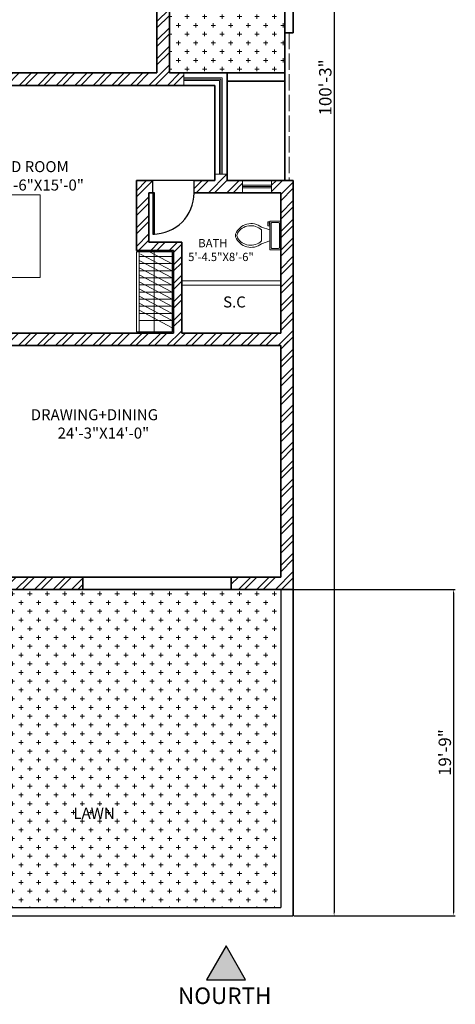
# Model space of a CAD drawing. Units: inches. Extents: x 839 to 1638, y 2998 to 4342.
# Tile 2 of 4: x 1321 to 1638, y 2998 to 3713. Entities that reach past the tile are written whole.
import ezdxf

# ---------------------------------------------------------------- set-up
doc = ezdxf.new("R2010")
doc.units = ezdxf.units.IN
doc.linetypes.add('ACAD_ISO02W100', pattern=[15, 12, -3])
for name, color, linetype, lineweight in [('A-ANNO-DIMS', 2, 'Continuous', 18), ('A-ANNO-SYMB', 7, 'Continuous', 25), ('A-AREA-IDEN', 7, 'Continuous', 18), ('A-DOOR', 4, 'Continuous', 25), ('A-DOOR-JAMB', 7, 'Continuous', 25), ('A-FLOR-CASE', 9, 'Continuous', 20), ('A-FLOR-CASE-PATT', 252, 'Continuous', 13), ('A-FLOR-FIXT', 9, 'Continuous', 18), ('A-FLOR-OVHD', 8, 'ACAD_ISO02W100', 18), ('A-FURN', 8, 'Continuous', 18), ('A-WALL', 7, 'Continuous', 35), ('A-WALL-PATT', 252, 'Continuous', 13), ('C-PROP', 7, 'Continuous', 30)]:
    doc.layers.add(name, color=color, linetype=linetype, lineweight=lineweight)
doc.layers.add('A-GLAZ', color=244, linetype='Continuous', lineweight=20, true_color=0x991b1e)
doc.layers.add('L-SITE-PATT', color=116, linetype='Continuous', lineweight=13, true_color=0x136734)
doc.styles.get("Standard").update_dxf_attribs({"font": 'arial.ttf'})
doc.dimstyles.new('ISO-25', dxfattribs={"dimtxt": 9, "dimasz": 2.5, "dimexe": 1.25, "dimexo": 0.625, "dimtad": 1, "dimlunit": 3, "dimtxsty": 'Standard', "dimcen": 2.5, "dimadec": 0, "dimazin": 0, "dimtfac": 1, "dimtmove": 0, "dimatfit": 3, "dimfxl": 1, "dimarcsym": 0})

# ---------------------------------------------------------------- blocks, each defined once
blk = doc.blocks.new('*U4')
for p, q in [((0, 0), (0, 6)), ((40, 0), (40, 6))]:
    blk.add_line(p, q)
blk.add_lwpolyline([(0, 0), (0, -40), (1.75, -40), (1.75, 0)], close=True)
blk.add_arc((0, 0), 40, 270, 0)
blk = doc.blocks.new('*U15')
for p, q in [((9.5, -6), (9.5, -2)), ((-10, -8.5), (-8, -8.5)), ((-10, -9.5), (-10, -8.5)), ((-7, -9.5), (-10, -9.5)), ((-8, -8.5), (-8, -8)), ((-7, -8), (-7, -9.5)), ((-4, -8), (-6, -14)), ((4, -14), (-4, -14)), ((4, -8), (6, -14))]:
    blk.add_line(p, q)
blk.add_lwpolyline([(10.5, -8), (10.5, 0), (-10.5, 0), (-10.5, -8)], close=True)
for points in [[(-9.5, -2), (-9.5, -6)], [(8.5, -1), (-8.5, -1)], [(-8.5, -7), (8.5, -7)]]:
    blk.add_lwpolyline(points)
for centre, radius, start, end in [((-8.62, -1.88), 0.884, 81.8699, 188.1301), ((-8.62, -6.12), 0.884, 171.8699, 278.1301), ((8.62, -1.88), 0.884, 351.8699, 98.1301), ((8.62, -6.12), 0.884, 261.8699, 8.1301), ((3.52, -21.58), 12.17, 141.46911, 247.97143), ((4.2, -21.82), 11.33, 136.36773, 238.94682), ((-3.52, -21.58), 12.17, 292.02843, 38.53071), ((-4.2, -21.82), 11.33, 301.05301, 43.63209), ((0, -27.88), 4, 245.73182, 294.26817), ((0, -29), 4, 254.86053, 285.13947)]:
    blk.add_arc(centre, radius, start, end)
blk = doc.blocks.new('Bed - Queen')
for p, q in [((0, -80.00003), (0, 0)), ((0, 0), (59.99999, 0)), ((59.99999, 0), (59.99999, -80.00003)), ((7.99999, -1.2), (28.79998, -1.2)), ((7.99999, -14.4), (7.99999, -1.2)), ((28.79998, -1.2), (28.79998, -14.4)), ((31.19999, -1.2), (51.99999, -1.2)), ((31.19999, -14.4), (31.19999, -1.2)), ((51.99999, -1.2), (51.99999, -16.4)), ((0, -14.4), (44.8, -14.4)), ((44.8, -16.8), (0, -16.8)), ((59.99999, -29.6), (44.8, -14.4)), ((44.8, -14.4), (44.8, -29.6)), ((51.99999, -16.4), (46.79936, -16.4)), ((44.8, -29.6), (59.99999, -29.6)), ((59.99999, -80.00003), (0, -80.00003))]:
    blk.add_line(p, q)
blk = doc.blocks.new('*D21')
at = {"layer": 'A-ANNO-DIMS', "color": 0, "lineweight": -2, "transparency": 16777216}
for p, q in [((1520.79, 4264.84), (1551.14, 4264.84)), ((1549.89, 4262.34), (1549.89, 3064.34)), ((1520.79, 3061.84), (1551.14, 3061.84))]:
    blk.add_line(p, q, dxfattribs=at)
at = {"layer": 'A-ANNO-DIMS', "color": 0, "transparency": 16777216}
for points in [[(1549.48, 4262.34), (1550.31, 4262.34), (1549.89, 4264.84)], [(1549.48, 3064.34), (1550.31, 3064.34), (1549.89, 3061.84)]]:
    blk.add_solid(points, dxfattribs=at)
at = {"layer": 'Defpoints', "color": 0, "transparency": 16777216}
for p in [(1520.17, 4264.84), (1520.17, 3061.84), (1549.89, 3061.84)]:
    blk.add_point(p, dxfattribs=at)
at = {"layer": 'A-ANNO-DIMS', "color": 0, "transparency": 16777216, "insert": (1544.67, 3663.34), "char_height": 9, "attachment_point": 5, "rotation": 90}
blk.add_mtext('100\'-3"', dxfattribs=at)
blk = doc.blocks.new('WIN-21x9')
for p, q in [((0, 5.5), (21, 5.5)), ((0, 4.5), (21, 4.5)), ((0, 3.5), (21, 3.5))]:
    blk.add_line(p, q)
blk.add_lwpolyline([(0, 9), (21, 9), (21, 0), (0, 0)], close=True)
blk = doc.blocks.new('*D51')
at = {"layer": 'A-ANNO-DIMS', "color": 0, "lineweight": -2, "transparency": 16777216}
for p, q in [((1520.79, 3298.84), (1638.02, 3298.84)), ((1636.77, 3296.34), (1636.77, 3064.34)), ((1520.79, 3061.84), (1638.02, 3061.84))]:
    blk.add_line(p, q, dxfattribs=at)
at = {"layer": 'A-ANNO-DIMS', "color": 0, "transparency": 16777216}
for points in [[(1636.35, 3296.34), (1637.19, 3296.34), (1636.77, 3298.84)], [(1636.35, 3064.34), (1637.19, 3064.34), (1636.77, 3061.84)]]:
    blk.add_solid(points, dxfattribs=at)
at = {"layer": 'Defpoints', "color": 0, "transparency": 16777216}
for p in [(1520.17, 3298.84), (1520.17, 3061.84), (1636.77, 3061.84)]:
    blk.add_point(p, dxfattribs=at)
at = {"layer": 'A-ANNO-DIMS', "color": 0, "transparency": 16777216, "insert": (1631.55, 3180.34), "char_height": 9, "attachment_point": 5, "rotation": 90}
blk.add_mtext('19\'-9"', dxfattribs=at)

msp = doc.modelspace()

# ---------------------------------------------------------------- hatches: boundary and pattern name
at = {"layer": 'A-ANNO-SYMB'}
h = msp.add_hatch(color=256, dxfattribs=at)
h.dxf.hatch_style = 1
h.paths.add_polyline_path([(1471.353, 3040.045), (1457.144, 3015.434), (1485.562, 3015.434)])
at = {"layer": 'A-FLOR-CASE-PATT'}
h = msp.add_hatch(dxfattribs=at)
h.set_pattern_fill('ANSI31', color=256, scale=1.438559, angle=107.2466, style=0)
h.paths.add_polyline_path([(1408.169, 3498.465), (1432.169, 3485.836), (1432.169, 3537.447), (1419.802, 3543.955), (1409.993, 3543.955), (1408.169, 3539.754)])
h = msp.add_hatch(dxfattribs=at)
h.set_pattern_fill('ANSI31', color=256, scale=1.625564, angle=-45, style=0)
h.paths.add_polyline_path([(1408.169, 3490.997), (1432.169, 3490.997), (1432.169, 3542.609), (1408.169, 3542.609)])
at = {"layer": 'A-WALL-PATT'}
h = msp.add_hatch(dxfattribs=at)
h.set_pattern_fill('ANSI32', color=256)
h.paths.add_polyline_path([(1440.674, 3673.836), (1430.169, 3673.836), (1430.169, 3724.836), (1421.169, 3724.836), (1421.169, 3673.836), (1209.669, 3673.836), (1209.669, 3670.236), (1209.669, 3664.836), (1247.169, 3664.836), (1247.169, 3661.836), (1252.569, 3661.836), (1256.169, 3661.836), (1256.169, 3664.836), (1440.674, 3664.836)])
h.paths.add_polyline_path([(1137.669, 3673.836), (1100.169, 3673.836), (1100.169, 3733.836), (1091.169, 3733.836), (1067.169, 3733.836), (1067.169, 3727.836), (1091.169, 3727.836), (1091.169, 3640.836), (971.169, 3640.836), (971.169, 3694.836), (962.169, 3694.836), (962.169, 3640.836), (896.169, 3640.836), (896.169, 3628.836), (905.169, 3628.836), (905.169, 3631.836), (1091.169, 3631.836), (1091.169, 3628.836), (1100.169, 3628.836), (1100.169, 3664.836), (1137.669, 3664.836)])
h.paths.add_polyline_path([(1256.169, 3625.836), (1247.169, 3625.836), (1247.169, 3491.75), (1237.967, 3478.332), (1245.508, 3473.161), (1247.169, 3475.836), (1520.169, 3475.836), (1520.169, 3595.836), (1504.368, 3595.836), (1504.368, 3586.836), (1511.169, 3586.836), (1511.169, 3484.836), (1439.169, 3484.836), (1439.169, 3550.955), (1415.169, 3550.955), (1415.169, 3586.836), (1418.169, 3586.836), (1418.169, 3595.836), (1406.169, 3595.836), (1406.169, 3544.955), (1433.169, 3544.955), (1433.169, 3484.836), (1406.169, 3484.836), (1256.169, 3484.836)])
h.paths.add_polyline_path([(1483.368, 3595.836), (1472.169, 3595.836), (1472.169, 3600.336), (1463.169, 3600.336), (1463.169, 3595.836), (1448.169, 3595.836), (1448.169, 3586.836), (1483.368, 3586.836)], flags=17)
h.paths.add_polyline_path([(1220.169, 3432.336), (1210.822, 3438.745), (1206.427, 3432.336), (1179.669, 3432.336), (1179.669, 3423.336), (1211.169, 3423.336), (1211.169, 3298.836), (1367.169, 3298.836), (1367.169, 3307.836), (1220.169, 3307.836)])
h.paths.add_polyline_path([(1041.669, 3532.086), (1058.169, 3532.086), (1058.169, 3541.086), (1032.669, 3541.086), (1032.669, 3432.336), (905.169, 3432.336), (905.169, 3470.704), (896.169, 3470.704), (896.169, 3423.336), (1055.555, 3423.336), (1055.555, 3432.336), (1041.669, 3432.336)])
h.paths.add_polyline_path([(1100.169, 3592.836), (1091.169, 3592.836), (1091.169, 3541.086), (1088.169, 3541.086), (1088.169, 3532.086), (1091.169, 3532.086), (1091.169, 3432.336), (1076.555, 3432.336), (1076.555, 3423.336), (1100.169, 3423.336), (1107.669, 3423.336), (1107.669, 3432.336), (1100.169, 3432.336)])
h.paths.add_polyline_path([(905.169, 3592.836), (896.169, 3592.836), (896.169, 3566.704), (905.169, 3566.704)])
h.paths.add_polyline_path([(905.169, 3763.836), (896.169, 3763.836), (896.169, 3727.836), (962.169, 3727.836), (962.169, 3724.836), (971.169, 3724.836), (971.169, 3727.836), (1031.169, 3727.836), (1031.169, 3733.836), (905.169, 3733.836)])
h.paths.add_polyline_path([(1109.169, 3892.836), (1100.169, 3892.836), (1100.169, 3895.836), (1091.169, 3895.836), (1091.169, 3886.836), (905.169, 3886.836), (905.169, 3937.836), (896.169, 3937.836), (896.169, 3847.836), (905.169, 3847.836), (905.169, 3877.836), (1091.169, 3877.836), (1091.169, 3859.836), (1100.169, 3859.836), (1100.169, 3883.836), (1109.169, 3883.836)])
h.paths.add_polyline_path([(905.169, 4162.836), (962.764, 4162.836), (962.764, 4171.836), (896.169, 4171.836), (896.169, 3997.836), (905.169, 3997.836), (905.169, 4048.836), (1010.169, 4048.836), (1010.169, 4054.836), (1007.169, 4054.836), (1007.169, 4057.836), (1001.169, 4057.836), (1001.169, 4054.836), (905.169, 4054.836)])
h.paths.add_polyline_path([(1152.669, 4171.836), (983.764, 4171.836), (983.764, 4162.836), (1001.169, 4162.836), (1001.169, 4087.836), (1007.169, 4087.836), (1007.169, 4162.836), (1073.169, 4162.836), (1073.169, 4054.836), (1046.169, 4054.836), (1046.169, 4048.836), (1091.169, 4048.836), (1091.169, 3931.836), (1100.169, 3931.836), (1100.169, 3991.836), (1103.169, 3991.836), (1103.169, 4000.836), (1100.169, 4000.836), (1100.169, 4054.836), (1079.169, 4054.836), (1079.169, 4162.836), (1152.669, 4162.836)])
h.paths.add_polyline_path([(1336.119, 4171.836), (1212.669, 4171.836), (1212.669, 4162.836), (1286.169, 4162.836), (1286.169, 4159.836), (1295.169, 4159.836), (1295.169, 4162.836), (1336.119, 4162.836)], flags=17)
h.paths.add_polyline_path([(1295.169, 4129.836), (1286.169, 4129.836), (1286.169, 4000.836), (1139.169, 4000.836), (1139.169, 3991.836), (1286.169, 3991.836), (1286.169, 3931.836), (1295.169, 3931.836), (1295.169, 4072.836), (1451.169, 4072.836), (1451.169, 4078.836), (1421.169, 4078.836), (1421.169, 4141.836), (1452.669, 4141.836), (1452.669, 4147.836), (1424.169, 4147.836), (1397.169, 4171.836), (1397.169, 4199.532), (1388.169, 4199.532), (1388.169, 4171.836), (1357.119, 4171.836), (1357.119, 4162.836), (1398.069, 4162.836), (1415.169, 4147.29), (1415.169, 4078.836), (1295.169, 4078.836)])
h.paths.add_polyline_path([(1442.169, 3892.836), (1295.169, 3892.836), (1295.169, 3895.836), (1286.169, 3895.836), (1286.169, 3892.836), (1277.169, 3892.836), (1277.169, 3883.836), (1421.169, 3883.836), (1421.169, 3832.836), (1430.169, 3832.836), (1430.169, 3883.836), (1442.169, 3883.836)])
h.paths.add_polyline_path([(1520.169, 4264.836), (1388.169, 4264.836), (1388.169, 4220.532), (1397.169, 4220.532), (1397.169, 4255.836), (1511.169, 4255.836), (1511.169, 4147.836), (1482.669, 4147.836), (1482.669, 4141.836), (1511.169, 4141.836), (1511.169, 4078.836), (1481.169, 4078.836), (1481.169, 4072.836), (1511.169, 4072.836), (1511.169, 3892.836), (1502.169, 3892.836), (1502.169, 3883.836), (1514.169, 3883.836), (1514.169, 3724.836), (1520.169, 3724.836)])
h.paths.add_polyline_path([(1319.528, 4099.601), (1381.705, 4099.601), (1381.705, 4129.453), (1319.528, 4129.453)], flags=25)
h = msp.add_hatch(dxfattribs=at)
h.set_pattern_fill('ANSI32', color=256)
h.paths.add_polyline_path([(1520.169, 3595.836), (1504.368, 3595.836), (1504.368, 3586.836), (1511.169, 3586.836), (1511.169, 3484.836), (1439.169, 3484.836), (1439.169, 3550.955), (1415.169, 3550.955), (1415.169, 3586.836), (1418.169, 3586.836), (1418.169, 3595.836), (1406.169, 3595.836), (1406.169, 3544.955), (1433.169, 3544.955), (1433.169, 3484.836), (1406.169, 3484.836), (1256.169, 3484.836), (1256.169, 3625.836), (1247.169, 3625.836), (1247.169, 3491.75), (1237.967, 3478.332), (1245.508, 3473.161), (1247.169, 3475.836), (1511.169, 3475.836), (1511.169, 3307.836), (1475.169, 3307.836), (1475.169, 3298.836), (1520.169, 3298.836)])
at = {"layer": 'L-SITE-PATT'}
h = msp.add_hatch(dxfattribs=at)
h.set_pattern_fill('CROSS', color=256)
h.paths.add_polyline_path([(1514.169, 3883.836), (1430.169, 3883.836), (1430.169, 3724.836), (1514.169, 3724.836)])
h.paths.add_polyline_path([(1514.169, 3718.836), (1430.169, 3718.836), (1430.169, 3673.836), (1514.169, 3673.836)])
h.paths.add_polyline_path([(1514.169, 3724.836), (1430.169, 3724.836), (1430.169, 3718.836), (1514.169, 3718.836)])
h.paths.add_polyline_path([(1436.251, 3779.553), (1499.144, 3779.553), (1499.144, 3809.372), (1436.251, 3809.372)], flags=24)
h = msp.add_hatch(dxfattribs=at)
h.set_pattern_fill('CROSS', color=256)
h.paths.add_polyline_path([(1511.169, 3298.836), (1221.169, 3298.836), (1221.169, 3222.336), (1094.996, 3222.336), (1094.996, 3067.836), (1511.169, 3067.836)])
h.paths.add_polyline_path([(1357.633, 3127.879), (1393.922, 3127.879), (1393.922, 3144.365), (1357.633, 3144.365)], flags=24)

# ---------------------------------------------------------------- linework, layer by layer
at = {"layer": 'A-ANNO-SYMB'}
msp.add_lwpolyline([(1471.353, 3040.045), (1457.144, 3015.434), (1485.562, 3015.434)], close=True, dxfattribs=at)
at = {"layer": 'A-DOOR'}
msp.add_line((1448.169, 3595.836), (1418.169, 3595.836), dxfattribs=at)
at = {"layer": 'A-DOOR-JAMB'}
for p, q in [((1418.169, 3586.836), (1418.169, 3595.836)), ((1448.169, 3586.836), (1448.169, 3595.836))]:
    msp.add_line(p, q, dxfattribs=at)
at = {"layer": 'A-FLOR-CASE'}
for p, q in [((1406.169, 3543.955), (1432.169, 3543.955)), ((1406.169, 3543.955), (1406.169, 3485.836)), ((1408.169, 3543.955), (1408.169, 3485.836)), ((1419.169, 3543.955), (1419.169, 3485.836)), ((1432.169, 3543.955), (1432.169, 3485.836)), ((1406.169, 3485.836), (1432.169, 3485.836))]:
    msp.add_line(p, q, dxfattribs=at)
at = {"layer": 'A-FLOR-FIXT'}
for p, q in [((1439.169, 3522.836), (1511.169, 3522.836)), ((1439.169, 3519.836), (1511.169, 3519.836))]:
    msp.add_line(p, q, dxfattribs=at)
at = {"layer": 'A-FLOR-OVHD'}
msp.add_line((1517.169, 3703.057), (1517.169, 3595.836), dxfattribs=at)
at = {"layer": 'A-GLAZ'}
for p, q in [((1440.674, 3670.336), (1468.669, 3670.336)), ((1440.674, 3669.336), (1467.669, 3669.336)), ((1440.674, 3668.336), (1466.669, 3668.336)), ((1466.669, 3668.336), (1466.669, 3600.336)), ((1467.669, 3669.336), (1467.669, 3600.336)), ((1468.669, 3670.336), (1468.669, 3600.336))]:
    msp.add_line(p, q, dxfattribs=at)
for points in [[(1461.674, 3664.836), (1440.674, 3664.836), (1440.674, 3673.836), (1461.674, 3673.836)], [(1472.169, 3660.336), (1472.169, 3600.336), (1463.169, 3600.336), (1463.169, 3660.336)]]:
    msp.add_lwpolyline(points, dxfattribs=at)
at = {"layer": 'A-WALL'}
for p, q in [((1520.169, 4264.836), (1520.169, 3703.057)), ((1421.169, 3883.836), (1421.169, 3673.836)), ((1430.169, 3883.836), (1430.169, 3673.836)), ((1514.169, 3883.836), (1514.169, 3595.836)), ((1514.169, 3703.057), (1520.169, 3703.057)), ((1209.669, 3673.836), (1421.169, 3673.836)), ((1430.169, 3673.836), (1514.169, 3673.836)), ((1472.169, 3673.836), (1472.169, 3595.836)), ((1472.169, 3667.836), (1514.169, 3667.836)), ((1256.169, 3664.836), (1463.169, 3664.836)), ((1463.169, 3664.836), (1463.169, 3595.836)), ((1406.169, 3595.836), (1406.169, 3544.955)), ((1406.169, 3595.836), (1418.169, 3595.836)), ((1448.169, 3595.836), (1463.169, 3595.836)), ((1472.169, 3595.836), (1520.169, 3595.836)), ((1520.169, 3595.836), (1520.169, 3061.836)), ((1415.169, 3586.836), (1415.169, 3550.955)), ((1415.169, 3586.836), (1418.169, 3586.836)), ((1448.169, 3586.836), (1511.169, 3586.836)), ((1511.169, 3586.836), (1511.169, 3484.836)), ((1415.169, 3550.955), (1439.169, 3550.955)), ((1439.169, 3550.955), (1439.169, 3484.836)), ((1406.169, 3544.955), (1433.169, 3544.955)), ((1433.169, 3544.955), (1433.169, 3484.836)), ((1256.169, 3484.836), (1406.169, 3484.836)), ((1406.169, 3484.836), (1433.169, 3484.836)), ((1439.169, 3484.836), (1511.169, 3484.836)), ((1247.169, 3475.836), (1511.169, 3475.836)), ((1511.169, 3475.836), (1511.169, 3307.836)), ((1220.169, 3307.836), (1511.169, 3307.836)), ((1367.169, 3307.836), (1367.169, 3298.836)), ((1475.169, 3307.836), (1475.169, 3298.836)), ((1211.169, 3298.836), (1520.169, 3298.836))]:
    msp.add_line(p, q, dxfattribs=at)
at = {"layer": 'C-PROP'}
for p, q in [((1511.169, 3298.836), (1511.169, 3067.836)), ((1094.996, 3067.836), (1511.169, 3067.836)), ((1094.996, 3061.836), (1520.169, 3061.836))]:
    msp.add_line(p, q, dxfattribs=at)

# ---------------------------------------------------------------- block references
at = {"layer": 'A-DOOR', "xscale": 0.7499999999999982, "yscale": 0.7499999999999982, "zscale": 0.7499999999999982}
msp.add_blockref('*U4', (1418.169, 3586.836), dxfattribs=at)
at = {"layer": 'A-FLOR-FIXT', "rotation": 270}
msp.add_blockref('*U15', (1511.169, 3555.837), dxfattribs=at)
at = {"layer": 'A-FURN', "xscale": -1, "rotation": 90}
msp.add_blockref('Bed - Queen', (1256.169, 3585.336), dxfattribs=at)
at = {"layer": 'A-GLAZ'}
msp.add_blockref('WIN-21x9', (1483.368, 3586.836), dxfattribs=at)

# ---------------------------------------------------------------- texts
at = {"layer": 'A-ANNO-SYMB', "insert": (1436.459, 3009.781), "char_height": 12, "attachment_point": 1}
msp.add_mtext_dynamic_manual_height_columns('NOURTH', width=76.099, gutter_width=12.5, heights=[0], dxfattribs=at)
at = {"layer": 'A-AREA-IDEN', "attachment_point": 1}
for s, width, insert, char_height in [('BED ROOM \\P12\'-6"X15\'-0"', 64.46402, (1301.467, 3609.819), 8), ('    BATH\\P5\'-4.5"X8\'-6"', 45.94447, (1443.857, 3553.275), 6), ('S.C', 16.07573, (1469.227, 3511.567), 8), ('DRAWING+DINING\\P        24\'-3"X14\'-0"', 106.25868, (1329.386, 3429.693), 8), ('LAWN', 34.28643, (1360.451, 3140.248), 8)]:
    msp.add_mtext_dynamic_manual_height_columns(s, width=width, gutter_width=12.5, heights=[0], dxfattribs=dict(at, insert=insert, char_height=char_height))

# ---------------------------------------------------------------- dimensions: what is measured, and where the dimension line sits
at = {"layer": 'A-ANNO-DIMS'}
for base, p1, override, picture, middle in [((1549.893, 3061.836), (1520.169, 4264.836), {"dimclrd": 0, "dimclre": 0, "dimclrt": 0}, '*D21', (1544.67, 3663.336)), ((1636.769, 3061.836), (1520.169, 3298.836), {"dimdec": 1, "dimlfac": 1, "dimrnd": 0, "dimzin": 1, "dimdsep": 46, "dimlunit": 4, "dimfrac": 2}, '*D51', (1631.548, 3180.336))]:
    dim = msp.add_linear_dim(base=base, p1=p1, p2=(1520.169, 3061.836), angle=90, dimstyle='ISO-25', override=override, dxfattribs=at)
    dim.commit()
    dim.dimension.update_dxf_attribs({"geometry": picture, "text_midpoint": middle})

doc.saveas('drawing.dxf')
